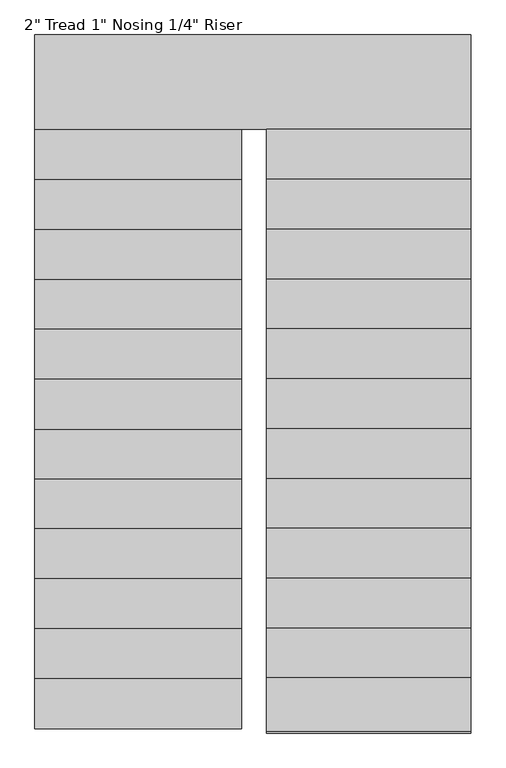
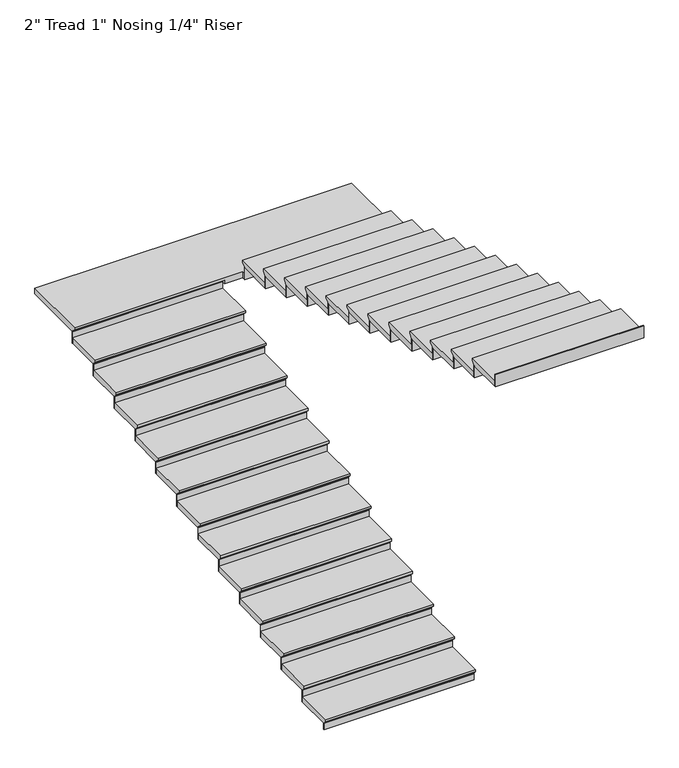
"""IFC4 building model written with IfcOpenShell, lengths in millimetres: stair flight geometry."""

from ifc_helpers import new_model, si_unit, origin, place, context, project, spatial, faceted_brep, source, transform, mapped, element, save


def stair_flight_ff411a25(model_context):
    return source(origin(), model_context, "Body", "Brep", [
        faceted_brep([(-2593.7381751, -9955.5916506, 9230.4576923), (-2593.7381751, -9955.5916506, 9249.5076923), (-3857.687215, -9955.5916506, 9249.5076923), (-3857.687215, -9955.5916506, 9230.4576923), (-2593.7381751, -9930.1916506, 9205.0576923), (-3857.687215, -9930.1916506, 9205.0576923), (-2593.7381751, -9619.0416506, 9249.5076923), (-3857.687215, -9619.0416506, 9249.5076923), (-3857.687215, -9930.1916506, 9198.7076923), (-3857.687215, -9619.0416506, 9198.7076923), (-2593.7381751, -9619.0416506, 9198.7076923), (-2593.7381751, -9930.1916506, 9198.7076923)], [[[0, 1, 2, 3]], [[4, 0, 3, 5]], [[2, 1, 6, 7]], [[8, 9, 10, 11]], [[2, 7, 9, 8, 5, 3]], [[8, 11, 4, 5]], [[6, 1, 0, 4, 11, 10]], [[7, 6, 10, 9]]]),
        faceted_brep([(-2593.7381751, -9930.1916506, 9198.7076923), (-2593.7381751, -9930.1916506, 9144.0), (-2593.7381751, -9923.8416506, 9144.0), (-2593.7381751, -9923.8416506, 9198.7076923), (-3857.687215, -9930.1916506, 9198.7076923), (-3857.687215, -9923.8416506, 9198.7076923), (-3857.687215, -9923.8416506, 9144.0), (-3857.687215, -9930.1916506, 9144.0)], [[[0, 1, 2, 3]], [[4, 5, 6, 7]], [[1, 0, 4, 7]], [[2, 1, 7, 6]], [[3, 2, 6, 5]], [[0, 3, 5, 4]]]),
        faceted_brep([(-2593.7381751, -9619.0416506, 9304.2153846), (-2593.7381751, -9619.0416506, 9198.7076923), (-2593.7381751, -9612.6916506, 9198.7076923), (-2593.7381751, -9612.6916506, 9304.2153846), (-3857.687215, -9619.0416506, 9304.2153846), (-3857.687215, -9612.6916506, 9304.2153846), (-3857.687215, -9612.6916506, 9198.7076923), (-3857.687215, -9619.0416506, 9198.7076923)], [[[0, 1, 2, 3]], [[4, 5, 6, 7]], [[1, 0, 4, 7]], [[2, 1, 7, 6]], [[3, 2, 6, 5]], [[0, 3, 5, 4]]]),
        faceted_brep([(-3857.687215, -9644.4416506, 9355.0153846), (-2593.7381751, -9644.4416506, 9355.0153846), (-2593.7381751, -9314.2416506, 9355.0153846), (-3857.687215, -9314.2416506, 9355.0153846), (-3857.687215, -9619.0416506, 9304.2153846), (-3857.687215, -9314.2416506, 9304.2153846), (-2593.7381751, -9314.2416506, 9304.2153846), (-2593.7381751, -9619.0416506, 9304.2153846), (-3857.687215, -9619.0416506, 9310.5653846), (-3857.687215, -9644.4416506, 9335.9653846), (-2593.7381751, -9619.0416506, 9310.5653846), (-2593.7381751, -9644.4416506, 9335.9653846)], [[[0, 1, 2, 3]], [[4, 5, 6, 7]], [[0, 3, 5, 4, 8, 9]], [[4, 7, 10, 8]], [[2, 1, 11, 10, 7, 6]], [[3, 2, 6, 5]], [[11, 1, 0, 9]], [[10, 11, 9, 8]]]),
        faceted_brep([(-2593.7381751, -9314.2416506, 9409.7230769), (-2593.7381751, -9314.2416506, 9304.2153846), (-2593.7381751, -9307.8916506, 9304.2153846), (-2593.7381751, -9307.8916506, 9409.7230769), (-3857.687215, -9314.2416506, 9409.7230769), (-3857.687215, -9307.8916506, 9409.7230769), (-3857.687215, -9307.8916506, 9304.2153846), (-3857.687215, -9314.2416506, 9304.2153846)], [[[0, 1, 2, 3]], [[4, 5, 6, 7]], [[1, 0, 4, 7]], [[2, 1, 7, 6]], [[3, 2, 6, 5]], [[0, 3, 5, 4]]]),
        faceted_brep([(-3857.687215, -9339.6416506, 9460.5230769), (-2593.7381751, -9339.6416506, 9460.5230769), (-2593.7381751, -9009.4416506, 9460.5230769), (-3857.687215, -9009.4416506, 9460.5230769), (-3857.687215, -9314.2416506, 9409.7230769), (-3857.687215, -9009.4416506, 9409.7230769), (-2593.7381751, -9009.4416506, 9409.7230769), (-2593.7381751, -9314.2416506, 9409.7230769), (-3857.687215, -9314.2416506, 9416.0730769), (-3857.687215, -9339.6416506, 9441.4730769), (-2593.7381751, -9314.2416506, 9416.0730769), (-2593.7381751, -9339.6416506, 9441.4730769)], [[[0, 1, 2, 3]], [[4, 5, 6, 7]], [[0, 3, 5, 4, 8, 9]], [[4, 7, 10, 8]], [[2, 1, 11, 10, 7, 6]], [[3, 2, 6, 5]], [[11, 1, 0, 9]], [[10, 11, 9, 8]]]),
        faceted_brep([(-2593.7381751, -9009.4416506, 9515.2307692), (-2593.7381751, -9009.4416506, 9409.7230769), (-2593.7381751, -9003.0916506, 9409.7230769), (-2593.7381751, -9003.0916506, 9515.2307692), (-3857.687215, -9009.4416506, 9515.2307692), (-3857.687215, -9003.0916506, 9515.2307692), (-3857.687215, -9003.0916506, 9409.7230769), (-3857.687215, -9009.4416506, 9409.7230769)], [[[0, 1, 2, 3]], [[4, 5, 6, 7]], [[1, 0, 4, 7]], [[2, 1, 7, 6]], [[3, 2, 6, 5]], [[0, 3, 5, 4]]]),
        faceted_brep([(-3857.687215, -9034.8416506, 9566.0307692), (-2593.7381751, -9034.8416506, 9566.0307692), (-2593.7381751, -8704.6416506, 9566.0307692), (-3857.687215, -8704.6416506, 9566.0307692), (-3857.687215, -9009.4416506, 9515.2307692), (-3857.687215, -8704.6416506, 9515.2307692), (-2593.7381751, -8704.6416506, 9515.2307692), (-2593.7381751, -9009.4416506, 9515.2307692), (-3857.687215, -9009.4416506, 9521.5807692), (-3857.687215, -9034.8416506, 9546.9807692), (-2593.7381751, -9009.4416506, 9521.5807692), (-2593.7381751, -9034.8416506, 9546.9807692)], [[[0, 1, 2, 3]], [[4, 5, 6, 7]], [[0, 3, 5, 4, 8, 9]], [[4, 7, 10, 8]], [[2, 1, 11, 10, 7, 6]], [[3, 2, 6, 5]], [[11, 1, 0, 9]], [[10, 11, 9, 8]]]),
        faceted_brep([(-2593.7381751, -8704.6416506, 9620.7384615), (-2593.7381751, -8704.6416506, 9515.2307692), (-2593.7381751, -8698.2916506, 9515.2307692), (-2593.7381751, -8698.2916506, 9620.7384615), (-3857.687215, -8704.6416506, 9620.7384615), (-3857.687215, -8698.2916506, 9620.7384615), (-3857.687215, -8698.2916506, 9515.2307692), (-3857.687215, -8704.6416506, 9515.2307692)], [[[0, 1, 2, 3]], [[4, 5, 6, 7]], [[1, 0, 4, 7]], [[2, 1, 7, 6]], [[3, 2, 6, 5]], [[0, 3, 5, 4]]]),
        faceted_brep([(-3857.687215, -8730.0416506, 9671.5384615), (-2593.7381751, -8730.0416506, 9671.5384615), (-2593.7381751, -8399.8416506, 9671.5384615), (-3857.687215, -8399.8416506, 9671.5384615), (-3857.687215, -8704.6416506, 9620.7384615), (-3857.687215, -8399.8416506, 9620.7384615), (-2593.7381751, -8399.8416506, 9620.7384615), (-2593.7381751, -8704.6416506, 9620.7384615), (-3857.687215, -8704.6416506, 9627.0884615), (-3857.687215, -8730.0416506, 9652.4884615), (-2593.7381751, -8704.6416506, 9627.0884615), (-2593.7381751, -8730.0416506, 9652.4884615)], [[[0, 1, 2, 3]], [[4, 5, 6, 7]], [[0, 3, 5, 4, 8, 9]], [[4, 7, 10, 8]], [[2, 1, 11, 10, 7, 6]], [[3, 2, 6, 5]], [[11, 1, 0, 9]], [[10, 11, 9, 8]]]),
        faceted_brep([(-2593.7381751, -8399.8416506, 9726.2461538), (-2593.7381751, -8399.8416506, 9620.7384615), (-2593.7381751, -8393.4916506, 9620.7384615), (-2593.7381751, -8393.4916506, 9726.2461538), (-3857.687215, -8399.8416506, 9726.2461538), (-3857.687215, -8393.4916506, 9726.2461538), (-3857.687215, -8393.4916506, 9620.7384615), (-3857.687215, -8399.8416506, 9620.7384615)], [[[0, 1, 2, 3]], [[4, 5, 6, 7]], [[1, 0, 4, 7]], [[2, 1, 7, 6]], [[3, 2, 6, 5]], [[0, 3, 5, 4]]]),
        faceted_brep([(-3857.687215, -8425.2416506, 9777.0461538), (-2593.7381751, -8425.2416506, 9777.0461538), (-2593.7381751, -8098.2166506, 9777.0461538), (-3857.687215, -8098.2166506, 9777.0461538), (-3857.687215, -8399.8416506, 9726.2461538), (-3857.687215, -8098.2166506, 9726.2461538), (-2593.7381751, -8098.2166506, 9726.2461538), (-2593.7381751, -8399.8416506, 9726.2461538), (-3857.687215, -8399.8416506, 9732.5961538), (-3857.687215, -8425.2416506, 9757.9961538), (-2593.7381751, -8399.8416506, 9732.5961538), (-2593.7381751, -8425.2416506, 9757.9961538)], [[[0, 1, 2, 3]], [[4, 5, 6, 7]], [[0, 3, 5, 4, 8, 9]], [[4, 7, 10, 8]], [[2, 1, 11, 10, 7, 6]], [[3, 2, 6, 5]], [[11, 1, 0, 9]], [[10, 11, 9, 8]]]),
        faceted_brep([(-2593.7381751, -8098.2166506, 9831.7538462), (-2593.7381751, -8098.2166506, 9726.2461538), (-2593.7381751, -8091.8666506, 9726.2461538), (-2593.7381751, -8091.8666506, 9831.7538462), (-3857.687215, -8098.2166506, 9831.7538462), (-3857.687215, -8091.8666506, 9831.7538462), (-3857.687215, -8091.8666506, 9726.2461538), (-3857.687215, -8098.2166506, 9726.2461538)], [[[0, 1, 2, 3]], [[4, 5, 6, 7]], [[1, 0, 4, 7]], [[2, 1, 7, 6]], [[3, 2, 6, 5]], [[0, 3, 5, 4]]]),
        faceted_brep([(-3857.687215, -8123.6166506, 9882.5538462), (-2593.7381751, -8123.6166506, 9882.5538462), (-2593.7381751, -7790.2416506, 9882.5538462), (-3857.687215, -7790.2416506, 9882.5538462), (-3857.687215, -8098.2166506, 9831.7538462), (-3857.687215, -7790.2416506, 9831.7538462), (-2593.7381751, -7790.2416506, 9831.7538462), (-2593.7381751, -8098.2166506, 9831.7538462), (-3857.687215, -8098.2166506, 9838.1038462), (-3857.687215, -8123.6166506, 9863.5038462), (-2593.7381751, -8098.2166506, 9838.1038462), (-2593.7381751, -8123.6166506, 9863.5038462)], [[[0, 1, 2, 3]], [[4, 5, 6, 7]], [[0, 3, 5, 4, 8, 9]], [[4, 7, 10, 8]], [[2, 1, 11, 10, 7, 6]], [[3, 2, 6, 5]], [[11, 1, 0, 9]], [[10, 11, 9, 8]]]),
        faceted_brep([(-2593.7381751, -7790.2416506, 9937.2615385), (-2593.7381751, -7790.2416506, 9831.7538462), (-2593.7381751, -7783.8916506, 9831.7538462), (-2593.7381751, -7783.8916506, 9937.2615385), (-3857.687215, -7790.2416506, 9937.2615385), (-3857.687215, -7783.8916506, 9937.2615385), (-3857.687215, -7783.8916506, 9831.7538462), (-3857.687215, -7790.2416506, 9831.7538462)], [[[0, 1, 2, 3]], [[4, 5, 6, 7]], [[1, 0, 4, 7]], [[2, 1, 7, 6]], [[3, 2, 6, 5]], [[0, 3, 5, 4]]]),
        faceted_brep([(-3857.687215, -7815.6416506, 9988.0615385), (-2593.7381751, -7815.6416506, 9988.0615385), (-2593.7381751, -7485.4416506, 9988.0615385), (-3857.687215, -7485.4416506, 9988.0615385), (-3857.687215, -7790.2416506, 9937.2615385), (-3857.687215, -7485.4416506, 9937.2615385), (-2593.7381751, -7485.4416506, 9937.2615385), (-2593.7381751, -7790.2416506, 9937.2615385), (-3857.687215, -7790.2416506, 9943.6115385), (-3857.687215, -7815.6416506, 9969.0115385), (-2593.7381751, -7790.2416506, 9943.6115385), (-2593.7381751, -7815.6416506, 9969.0115385)], [[[0, 1, 2, 3]], [[4, 5, 6, 7]], [[0, 3, 5, 4, 8, 9]], [[4, 7, 10, 8]], [[2, 1, 11, 10, 7, 6]], [[3, 2, 6, 5]], [[11, 1, 0, 9]], [[10, 11, 9, 8]]]),
        faceted_brep([(-2593.7381751, -7485.4416506, 10042.7692308), (-2593.7381751, -7485.4416506, 9937.2615385), (-2593.7381751, -7479.0916506, 9937.2615385), (-2593.7381751, -7479.0916506, 10042.7692308), (-3857.687215, -7485.4416506, 10042.7692308), (-3857.687215, -7479.0916506, 10042.7692308), (-3857.687215, -7479.0916506, 9937.2615385), (-3857.687215, -7485.4416506, 9937.2615385)], [[[0, 1, 2, 3]], [[4, 5, 6, 7]], [[1, 0, 4, 7]], [[2, 1, 7, 6]], [[3, 2, 6, 5]], [[0, 3, 5, 4]]]),
        faceted_brep([(-3857.687215, -7510.8416506, 10093.5692308), (-2593.7381751, -7510.8416506, 10093.5692308), (-2593.7381751, -7180.6416506, 10093.5692308), (-3857.687215, -7180.6416506, 10093.5692308), (-3857.687215, -7485.4416506, 10042.7692308), (-3857.687215, -7180.6416506, 10042.7692308), (-2593.7381751, -7180.6416506, 10042.7692308), (-2593.7381751, -7485.4416506, 10042.7692308), (-3857.687215, -7485.4416506, 10049.1192308), (-3857.687215, -7510.8416506, 10074.5192308), (-2593.7381751, -7485.4416506, 10049.1192308), (-2593.7381751, -7510.8416506, 10074.5192308)], [[[0, 1, 2, 3]], [[4, 5, 6, 7]], [[0, 3, 5, 4, 8, 9]], [[4, 7, 10, 8]], [[2, 1, 11, 10, 7, 6]], [[3, 2, 6, 5]], [[11, 1, 0, 9]], [[10, 11, 9, 8]]]),
        faceted_brep([(-2593.7381751, -7180.6416506, 10148.2769231), (-2593.7381751, -7180.6416506, 10042.7692308), (-2593.7381751, -7174.2916506, 10042.7692308), (-2593.7381751, -7174.2916506, 10148.2769231), (-3857.687215, -7180.6416506, 10148.2769231), (-3857.687215, -7174.2916506, 10148.2769231), (-3857.687215, -7174.2916506, 10042.7692308), (-3857.687215, -7180.6416506, 10042.7692308)], [[[0, 1, 2, 3]], [[4, 5, 6, 7]], [[1, 0, 4, 7]], [[2, 1, 7, 6]], [[3, 2, 6, 5]], [[0, 3, 5, 4]]]),
        faceted_brep([(-3857.687215, -7206.0416506, 10199.0769231), (-2593.7381751, -7206.0416506, 10199.0769231), (-2593.7381751, -6875.8416506, 10199.0769231), (-3857.687215, -6875.8416506, 10199.0769231), (-3857.687215, -7180.6416506, 10148.2769231), (-3857.687215, -6875.8416506, 10148.2769231), (-2593.7381751, -6875.8416506, 10148.2769231), (-2593.7381751, -7180.6416506, 10148.2769231), (-3857.687215, -7180.6416506, 10154.6269231), (-3857.687215, -7206.0416506, 10180.0269231), (-2593.7381751, -7180.6416506, 10154.6269231), (-2593.7381751, -7206.0416506, 10180.0269231)], [[[0, 1, 2, 3]], [[4, 5, 6, 7]], [[0, 3, 5, 4, 8, 9]], [[4, 7, 10, 8]], [[2, 1, 11, 10, 7, 6]], [[3, 2, 6, 5]], [[11, 1, 0, 9]], [[10, 11, 9, 8]]]),
        faceted_brep([(-2593.7381751, -6875.8416506, 10253.7846154), (-2593.7381751, -6875.8416506, 10148.2769231), (-2593.7381751, -6869.4916506, 10148.2769231), (-2593.7381751, -6869.4916506, 10253.7846154), (-3857.687215, -6875.8416506, 10253.7846154), (-3857.687215, -6869.4916506, 10253.7846154), (-3857.687215, -6869.4916506, 10148.2769231), (-3857.687215, -6875.8416506, 10148.2769231)], [[[0, 1, 2, 3]], [[4, 5, 6, 7]], [[1, 0, 4, 7]], [[2, 1, 7, 6]], [[3, 2, 6, 5]], [[0, 3, 5, 4]]]),
        faceted_brep([(-3857.687215, -6901.2416506, 10304.5846154), (-2593.7381751, -6901.2416506, 10304.5846154), (-2593.7381751, -6571.0416506, 10304.5846154), (-3857.687215, -6571.0416506, 10304.5846154), (-3857.687215, -6875.8416506, 10253.7846154), (-3857.687215, -6571.0416506, 10253.7846154), (-2593.7381751, -6571.0416506, 10253.7846154), (-2593.7381751, -6875.8416506, 10253.7846154), (-3857.687215, -6875.8416506, 10260.1346154), (-3857.687215, -6901.2416506, 10285.5346154), (-2593.7381751, -6875.8416506, 10260.1346154), (-2593.7381751, -6901.2416506, 10285.5346154)], [[[0, 1, 2, 3]], [[4, 5, 6, 7]], [[0, 3, 5, 4, 8, 9]], [[4, 7, 10, 8]], [[2, 1, 11, 10, 7, 6]], [[3, 2, 6, 5]], [[11, 1, 0, 9]], [[10, 11, 9, 8]]]),
        faceted_brep([(-2593.7381751, -6571.0416506, 10359.2923077), (-2593.7381751, -6571.0416506, 10253.7846154), (-2593.7381751, -6564.6916506, 10253.7846154), (-2593.7381751, -6564.6916506, 10359.2923077), (-3857.687215, -6571.0416506, 10359.2923077), (-3857.687215, -6564.6916506, 10359.2923077), (-3857.687215, -6564.6916506, 10253.7846154), (-3857.687215, -6571.0416506, 10253.7846154)], [[[0, 1, 2, 3]], [[4, 5, 6, 7]], [[1, 0, 4, 7]], [[2, 1, 7, 6]], [[3, 2, 6, 5]], [[0, 3, 5, 4]]]),
        faceted_brep([(-3857.687215, -6596.4416506, 10410.0923077), (-2593.7381751, -6596.4416506, 10410.0923077), (-2593.7381751, -6266.2416506, 10410.0923077), (-3857.687215, -6266.2416506, 10410.0923077), (-3857.687215, -6571.0416506, 10359.2923077), (-3857.687215, -6266.2416506, 10359.2923077), (-2593.7381751, -6266.2416506, 10359.2923077), (-2593.7381751, -6571.0416506, 10359.2923077), (-3857.687215, -6571.0416506, 10365.6423077), (-3857.687215, -6596.4416506, 10391.0423077), (-2593.7381751, -6571.0416506, 10365.6423077), (-2593.7381751, -6596.4416506, 10391.0423077)], [[[0, 1, 2, 3]], [[4, 5, 6, 7]], [[0, 3, 5, 4, 8, 9]], [[4, 7, 10, 8]], [[2, 1, 11, 10, 7, 6]], [[3, 2, 6, 5]], [[11, 1, 0, 9]], [[10, 11, 9, 8]]]),
        faceted_brep([(-2593.7381751, -6266.2416506, 10464.8), (-2593.7381751, -6266.2416506, 10359.2923077), (-2593.7381751, -6259.8916506, 10359.2923077), (-2593.7381751, -6259.8916506, 10464.8), (-3857.687215, -6266.2416506, 10464.8), (-3857.687215, -6259.8916506, 10464.8), (-3857.687215, -6259.8916506, 10359.2923077), (-3857.687215, -6266.2416506, 10359.2923077)], [[[0, 1, 2, 3]], [[4, 5, 6, 7]], [[1, 0, 4, 7]], [[2, 1, 7, 6]], [[3, 2, 6, 5]], [[0, 3, 5, 4]]]),
        faceted_brep([(-1190.687215, -6317.0416506, 10515.6), (-1190.687215, -5713.7916506, 10515.6), (-3857.687215, -5713.7916506, 10515.6), (-3857.687215, -6291.6416506, 10515.6), (-2441.3381751, -6291.6416506, 10515.6), (-2441.3381751, -6317.0416506, 10515.6), (-1190.687215, -5713.7916506, 10464.8), (-1190.687215, -6317.0416506, 10464.8), (-2441.3381751, -6317.0416506, 10464.8), (-2441.3381751, -6291.6416506, 10464.8), (-2593.7381751, -6291.6416506, 10464.8), (-2593.7381751, -6266.2416506, 10464.8), (-3857.687215, -6266.2416506, 10464.8), (-3857.687215, -5713.7916506, 10464.8), (-3857.687215, -6266.2416506, 10471.15), (-3857.687215, -6291.6416506, 10496.55), (-2593.7381751, -6266.2416506, 10471.15), (-2593.7381751, -6291.6416506, 10496.55)], [[[0, 1, 2, 3, 4, 5]], [[6, 7, 8, 9, 10, 11, 12, 13]], [[1, 0, 7, 6]], [[2, 1, 6, 13]], [[3, 2, 13, 12, 14, 15]], [[12, 11, 16, 14]], [[11, 10, 17, 16]], [[4, 3, 15, 17, 10, 9]], [[5, 4, 9, 8]], [[0, 5, 8, 7]], [[15, 14, 16, 17]]]),
        faceted_brep([(-2441.3381751, -6317.0416506, 10570.3076923), (-2441.3381751, -6317.0416506, 10464.8), (-2441.3381751, -6323.3916506, 10464.8), (-2441.3381751, -6323.3916506, 10570.3076923), (-1190.687215, -6317.0416506, 10570.3076923), (-1190.687215, -6323.3916506, 10570.3076923), (-1190.687215, -6323.3916506, 10464.8), (-1190.687215, -6317.0416506, 10464.8)], [[[0, 1, 2, 3]], [[4, 5, 6, 7]], [[1, 0, 4, 7]], [[2, 1, 7, 6]], [[3, 2, 6, 5]], [[0, 3, 5, 4]]]),
        faceted_brep([(-1190.687215, -6291.6416506, 10621.1076923), (-2441.3381751, -6291.6416506, 10621.1076923), (-2441.3381751, -6621.8416506, 10621.1076923), (-1190.687215, -6621.8416506, 10621.1076923), (-1190.687215, -6317.0416506, 10570.3076923), (-1190.687215, -6621.8416506, 10570.3076923), (-2441.3381751, -6621.8416506, 10570.3076923), (-2441.3381751, -6317.0416506, 10570.3076923), (-1190.687215, -6317.0416506, 10576.6576923), (-1190.687215, -6291.6416506, 10602.0576923), (-2441.3381751, -6317.0416506, 10576.6576923), (-2441.3381751, -6291.6416506, 10602.0576923)], [[[0, 1, 2, 3]], [[4, 5, 6, 7]], [[0, 3, 5, 4, 8, 9]], [[4, 7, 10, 8]], [[2, 1, 11, 10, 7, 6]], [[3, 2, 6, 5]], [[11, 1, 0, 9]], [[10, 11, 9, 8]]]),
        faceted_brep([(-2441.3381751, -6621.8416506, 10675.8153846), (-2441.3381751, -6621.8416506, 10570.3076923), (-2441.3381751, -6628.1916506, 10570.3076923), (-2441.3381751, -6628.1916506, 10675.8153846), (-1190.687215, -6621.8416506, 10675.8153846), (-1190.687215, -6628.1916506, 10675.8153846), (-1190.687215, -6628.1916506, 10570.3076923), (-1190.687215, -6621.8416506, 10570.3076923)], [[[0, 1, 2, 3]], [[4, 5, 6, 7]], [[1, 0, 4, 7]], [[2, 1, 7, 6]], [[3, 2, 6, 5]], [[0, 3, 5, 4]]]),
        faceted_brep([(-1190.687215, -6596.4416506, 10726.6153846), (-2441.3381751, -6596.4416506, 10726.6153846), (-2441.3381751, -6926.6416506, 10726.6153846), (-1190.687215, -6926.6416506, 10726.6153846), (-1190.687215, -6621.8416506, 10675.8153846), (-1190.687215, -6926.6416506, 10675.8153846), (-2441.3381751, -6926.6416506, 10675.8153846), (-2441.3381751, -6621.8416506, 10675.8153846), (-1190.687215, -6621.8416506, 10682.1653846), (-1190.687215, -6596.4416506, 10707.5653846), (-2441.3381751, -6621.8416506, 10682.1653846), (-2441.3381751, -6596.4416506, 10707.5653846)], [[[0, 1, 2, 3]], [[4, 5, 6, 7]], [[0, 3, 5, 4, 8, 9]], [[4, 7, 10, 8]], [[2, 1, 11, 10, 7, 6]], [[3, 2, 6, 5]], [[11, 1, 0, 9]], [[10, 11, 9, 8]]]),
        faceted_brep([(-2441.3381751, -6926.6416506, 10781.3230769), (-2441.3381751, -6926.6416506, 10675.8153846), (-2441.3381751, -6932.9916506, 10675.8153846), (-2441.3381751, -6932.9916506, 10781.3230769), (-1190.687215, -6926.6416506, 10781.3230769), (-1190.687215, -6932.9916506, 10781.3230769), (-1190.687215, -6932.9916506, 10675.8153846), (-1190.687215, -6926.6416506, 10675.8153846)], [[[0, 1, 2, 3]], [[4, 5, 6, 7]], [[1, 0, 4, 7]], [[2, 1, 7, 6]], [[3, 2, 6, 5]], [[0, 3, 5, 4]]]),
        faceted_brep([(-1190.687215, -6901.2416506, 10832.1230769), (-2441.3381751, -6901.2416506, 10832.1230769), (-2441.3381751, -7231.4416506, 10832.1230769), (-1190.687215, -7231.4416506, 10832.1230769), (-1190.687215, -6926.6416506, 10781.3230769), (-1190.687215, -7231.4416506, 10781.3230769), (-2441.3381751, -7231.4416506, 10781.3230769), (-2441.3381751, -6926.6416506, 10781.3230769), (-1190.687215, -6926.6416506, 10787.6730769), (-1190.687215, -6901.2416506, 10813.0730769), (-2441.3381751, -6926.6416506, 10787.6730769), (-2441.3381751, -6901.2416506, 10813.0730769)], [[[0, 1, 2, 3]], [[4, 5, 6, 7]], [[0, 3, 5, 4, 8, 9]], [[4, 7, 10, 8]], [[2, 1, 11, 10, 7, 6]], [[3, 2, 6, 5]], [[11, 1, 0, 9]], [[10, 11, 9, 8]]]),
        faceted_brep([(-2441.3381751, -7231.4416506, 10886.8307692), (-2441.3381751, -7231.4416506, 10781.3230769), (-2441.3381751, -7237.7916506, 10781.3230769), (-2441.3381751, -7237.7916506, 10886.8307692), (-1190.687215, -7231.4416506, 10886.8307692), (-1190.687215, -7237.7916506, 10886.8307692), (-1190.687215, -7237.7916506, 10781.3230769), (-1190.687215, -7231.4416506, 10781.3230769)], [[[0, 1, 2, 3]], [[4, 5, 6, 7]], [[1, 0, 4, 7]], [[2, 1, 7, 6]], [[3, 2, 6, 5]], [[0, 3, 5, 4]]]),
        faceted_brep([(-1190.687215, -7206.0416506, 10937.6307692), (-2441.3381751, -7206.0416506, 10937.6307692), (-2441.3381751, -7536.2416506, 10937.6307692), (-1190.687215, -7536.2416506, 10937.6307692), (-1190.687215, -7231.4416506, 10886.8307692), (-1190.687215, -7536.2416506, 10886.8307692), (-2441.3381751, -7536.2416506, 10886.8307692), (-2441.3381751, -7231.4416506, 10886.8307692), (-1190.687215, -7231.4416506, 10893.1807692), (-1190.687215, -7206.0416506, 10918.5807692), (-2441.3381751, -7231.4416506, 10893.1807692), (-2441.3381751, -7206.0416506, 10918.5807692)], [[[0, 1, 2, 3]], [[4, 5, 6, 7]], [[0, 3, 5, 4, 8, 9]], [[4, 7, 10, 8]], [[2, 1, 11, 10, 7, 6]], [[3, 2, 6, 5]], [[11, 1, 0, 9]], [[10, 11, 9, 8]]]),
        faceted_brep([(-2441.3381751, -7536.2416506, 10992.3384615), (-2441.3381751, -7536.2416506, 10886.8307692), (-2441.3381751, -7542.5916506, 10886.8307692), (-2441.3381751, -7542.5916506, 10992.3384615), (-1190.687215, -7536.2416506, 10992.3384615), (-1190.687215, -7542.5916506, 10992.3384615), (-1190.687215, -7542.5916506, 10886.8307692), (-1190.687215, -7536.2416506, 10886.8307692)], [[[0, 1, 2, 3]], [[4, 5, 6, 7]], [[1, 0, 4, 7]], [[2, 1, 7, 6]], [[3, 2, 6, 5]], [[0, 3, 5, 4]]]),
        faceted_brep([(-1190.687215, -7510.8416506, 11043.1384615), (-2441.3381751, -7510.8416506, 11043.1384615), (-2441.3381751, -7841.0416506, 11043.1384615), (-1190.687215, -7841.0416506, 11043.1384615), (-1190.687215, -7536.2416506, 10992.3384615), (-1190.687215, -7841.0416506, 10992.3384615), (-2441.3381751, -7841.0416506, 10992.3384615), (-2441.3381751, -7536.2416506, 10992.3384615), (-1190.687215, -7536.2416506, 10998.6884615), (-1190.687215, -7510.8416506, 11024.0884615), (-2441.3381751, -7536.2416506, 10998.6884615), (-2441.3381751, -7510.8416506, 11024.0884615)], [[[0, 1, 2, 3]], [[4, 5, 6, 7]], [[0, 3, 5, 4, 8, 9]], [[4, 7, 10, 8]], [[2, 1, 11, 10, 7, 6]], [[3, 2, 6, 5]], [[11, 1, 0, 9]], [[10, 11, 9, 8]]]),
        faceted_brep([(-2441.3381751, -7841.0416506, 11097.8461538), (-2441.3381751, -7841.0416506, 10992.3384615), (-2441.3381751, -7847.3916506, 10992.3384615), (-2441.3381751, -7847.3916506, 11097.8461538), (-1190.687215, -7841.0416506, 11097.8461538), (-1190.687215, -7847.3916506, 11097.8461538), (-1190.687215, -7847.3916506, 10992.3384615), (-1190.687215, -7841.0416506, 10992.3384615)], [[[0, 1, 2, 3]], [[4, 5, 6, 7]], [[1, 0, 4, 7]], [[2, 1, 7, 6]], [[3, 2, 6, 5]], [[0, 3, 5, 4]]]),
        faceted_brep([(-1190.687215, -7815.6416506, 11148.6461538), (-2441.3381751, -7815.6416506, 11148.6461538), (-2441.3381751, -8145.8416506, 11148.6461538), (-1190.687215, -8145.8416506, 11148.6461538), (-1190.687215, -7841.0416506, 11097.8461538), (-1190.687215, -8145.8416506, 11097.8461538), (-2441.3381751, -8145.8416506, 11097.8461538), (-2441.3381751, -7841.0416506, 11097.8461538), (-1190.687215, -7841.0416506, 11104.1961538), (-1190.687215, -7815.6416506, 11129.5961538), (-2441.3381751, -7841.0416506, 11104.1961538), (-2441.3381751, -7815.6416506, 11129.5961538)], [[[0, 1, 2, 3]], [[4, 5, 6, 7]], [[0, 3, 5, 4, 8, 9]], [[4, 7, 10, 8]], [[2, 1, 11, 10, 7, 6]], [[3, 2, 6, 5]], [[11, 1, 0, 9]], [[10, 11, 9, 8]]]),
        faceted_brep([(-2441.3381751, -8145.8416506, 11203.3538462), (-2441.3381751, -8145.8416506, 11097.8461538), (-2441.3381751, -8152.1916506, 11097.8461538), (-2441.3381751, -8152.1916506, 11203.3538462), (-1190.687215, -8145.8416506, 11203.3538462), (-1190.687215, -8152.1916506, 11203.3538462), (-1190.687215, -8152.1916506, 11097.8461538), (-1190.687215, -8145.8416506, 11097.8461538)], [[[0, 1, 2, 3]], [[4, 5, 6, 7]], [[1, 0, 4, 7]], [[2, 1, 7, 6]], [[3, 2, 6, 5]], [[0, 3, 5, 4]]]),
        faceted_brep([(-1190.687215, -8120.4416506, 11254.1538462), (-2441.3381751, -8120.4416506, 11254.1538462), (-2441.3381751, -8450.6416506, 11254.1538462), (-1190.687215, -8450.6416506, 11254.1538462), (-1190.687215, -8145.8416506, 11203.3538462), (-1190.687215, -8450.6416506, 11203.3538462), (-2441.3381751, -8450.6416506, 11203.3538462), (-2441.3381751, -8145.8416506, 11203.3538462), (-1190.687215, -8145.8416506, 11209.7038462), (-1190.687215, -8120.4416506, 11235.1038462), (-2441.3381751, -8145.8416506, 11209.7038462), (-2441.3381751, -8120.4416506, 11235.1038462)], [[[0, 1, 2, 3]], [[4, 5, 6, 7]], [[0, 3, 5, 4, 8, 9]], [[4, 7, 10, 8]], [[2, 1, 11, 10, 7, 6]], [[3, 2, 6, 5]], [[11, 1, 0, 9]], [[10, 11, 9, 8]]]),
        faceted_brep([(-2441.3381751, -8450.6416506, 11308.8615385), (-2441.3381751, -8450.6416506, 11203.3538462), (-2441.3381751, -8456.9916506, 11203.3538462), (-2441.3381751, -8456.9916506, 11308.8615385), (-1190.687215, -8450.6416506, 11308.8615385), (-1190.687215, -8456.9916506, 11308.8615385), (-1190.687215, -8456.9916506, 11203.3538462), (-1190.687215, -8450.6416506, 11203.3538462)], [[[0, 1, 2, 3]], [[4, 5, 6, 7]], [[1, 0, 4, 7]], [[2, 1, 7, 6]], [[3, 2, 6, 5]], [[0, 3, 5, 4]]]),
        faceted_brep([(-1190.687215, -8425.2416506, 11359.6615385), (-2441.3381751, -8425.2416506, 11359.6615385), (-2441.3381751, -8755.4416506, 11359.6615385), (-1190.687215, -8755.4416506, 11359.6615385), (-1190.687215, -8450.6416506, 11308.8615385), (-1190.687215, -8755.4416506, 11308.8615385), (-2441.3381751, -8755.4416506, 11308.8615385), (-2441.3381751, -8450.6416506, 11308.8615385), (-1190.687215, -8450.6416506, 11315.2115385), (-1190.687215, -8425.2416506, 11340.6115385), (-2441.3381751, -8450.6416506, 11315.2115385), (-2441.3381751, -8425.2416506, 11340.6115385)], [[[0, 1, 2, 3]], [[4, 5, 6, 7]], [[0, 3, 5, 4, 8, 9]], [[4, 7, 10, 8]], [[2, 1, 11, 10, 7, 6]], [[3, 2, 6, 5]], [[11, 1, 0, 9]], [[10, 11, 9, 8]]]),
        faceted_brep([(-2441.3381751, -8755.4416506, 11414.3692308), (-2441.3381751, -8755.4416506, 11308.8615385), (-2441.3381751, -8761.7916506, 11308.8615385), (-2441.3381751, -8761.7916506, 11414.3692308), (-1190.687215, -8755.4416506, 11414.3692308), (-1190.687215, -8761.7916506, 11414.3692308), (-1190.687215, -8761.7916506, 11308.8615385), (-1190.687215, -8755.4416506, 11308.8615385)], [[[0, 1, 2, 3]], [[4, 5, 6, 7]], [[1, 0, 4, 7]], [[2, 1, 7, 6]], [[3, 2, 6, 5]], [[0, 3, 5, 4]]]),
        faceted_brep([(-1190.687215, -8730.0416506, 11465.1692308), (-2441.3381751, -8730.0416506, 11465.1692308), (-2441.3381751, -9060.2416506, 11465.1692308), (-1190.687215, -9060.2416506, 11465.1692308), (-1190.687215, -8755.4416506, 11414.3692308), (-1190.687215, -9060.2416506, 11414.3692308), (-2441.3381751, -9060.2416506, 11414.3692308), (-2441.3381751, -8755.4416506, 11414.3692308), (-1190.687215, -8755.4416506, 11420.7192308), (-1190.687215, -8730.0416506, 11446.1192308), (-2441.3381751, -8755.4416506, 11420.7192308), (-2441.3381751, -8730.0416506, 11446.1192308)], [[[0, 1, 2, 3]], [[4, 5, 6, 7]], [[0, 3, 5, 4, 8, 9]], [[4, 7, 10, 8]], [[2, 1, 11, 10, 7, 6]], [[3, 2, 6, 5]], [[11, 1, 0, 9]], [[10, 11, 9, 8]]]),
        faceted_brep([(-2441.3381751, -9060.2416506, 11519.8769231), (-2441.3381751, -9060.2416506, 11414.3692308), (-2441.3381751, -9066.5916506, 11414.3692308), (-2441.3381751, -9066.5916506, 11519.8769231), (-1190.687215, -9060.2416506, 11519.8769231), (-1190.687215, -9066.5916506, 11519.8769231), (-1190.687215, -9066.5916506, 11414.3692308), (-1190.687215, -9060.2416506, 11414.3692308)], [[[0, 1, 2, 3]], [[4, 5, 6, 7]], [[1, 0, 4, 7]], [[2, 1, 7, 6]], [[3, 2, 6, 5]], [[0, 3, 5, 4]]]),
        faceted_brep([(-1190.687215, -9034.8416506, 11570.6769231), (-2441.3381751, -9034.8416506, 11570.6769231), (-2441.3381751, -9365.0416506, 11570.6769231), (-1190.687215, -9365.0416506, 11570.6769231), (-1190.687215, -9060.2416506, 11519.8769231), (-1190.687215, -9365.0416506, 11519.8769231), (-2441.3381751, -9365.0416506, 11519.8769231), (-2441.3381751, -9060.2416506, 11519.8769231), (-1190.687215, -9060.2416506, 11526.2269231), (-1190.687215, -9034.8416506, 11551.6269231), (-2441.3381751, -9060.2416506, 11526.2269231), (-2441.3381751, -9034.8416506, 11551.6269231)], [[[0, 1, 2, 3]], [[4, 5, 6, 7]], [[0, 3, 5, 4, 8, 9]], [[4, 7, 10, 8]], [[2, 1, 11, 10, 7, 6]], [[3, 2, 6, 5]], [[11, 1, 0, 9]], [[10, 11, 9, 8]]]),
        faceted_brep([(-2441.3381751, -9365.0416506, 11625.3846154), (-2441.3381751, -9365.0416506, 11519.8769231), (-2441.3381751, -9371.3916506, 11519.8769231), (-2441.3381751, -9371.3916506, 11625.3846154), (-1190.687215, -9365.0416506, 11625.3846154), (-1190.687215, -9371.3916506, 11625.3846154), (-1190.687215, -9371.3916506, 11519.8769231), (-1190.687215, -9365.0416506, 11519.8769231)], [[[0, 1, 2, 3]], [[4, 5, 6, 7]], [[1, 0, 4, 7]], [[2, 1, 7, 6]], [[3, 2, 6, 5]], [[0, 3, 5, 4]]]),
        faceted_brep([(-1190.687215, -9339.6416506, 11676.1846154), (-2441.3381751, -9339.6416506, 11676.1846154), (-2441.3381751, -9669.8416506, 11676.1846154), (-1190.687215, -9669.8416506, 11676.1846154), (-1190.687215, -9365.0416506, 11625.3846154), (-1190.687215, -9669.8416506, 11625.3846154), (-2441.3381751, -9669.8416506, 11625.3846154), (-2441.3381751, -9365.0416506, 11625.3846154), (-1190.687215, -9365.0416506, 11631.7346154), (-1190.687215, -9339.6416506, 11657.1346154), (-2441.3381751, -9365.0416506, 11631.7346154), (-2441.3381751, -9339.6416506, 11657.1346154)], [[[0, 1, 2, 3]], [[4, 5, 6, 7]], [[0, 3, 5, 4, 8, 9]], [[4, 7, 10, 8]], [[2, 1, 11, 10, 7, 6]], [[3, 2, 6, 5]], [[11, 1, 0, 9]], [[10, 11, 9, 8]]]),
        faceted_brep([(-2441.3381751, -9669.8416506, 11730.8923077), (-2441.3381751, -9669.8416506, 11625.3846154), (-2441.3381751, -9676.1916506, 11625.3846154), (-2441.3381751, -9676.1916506, 11730.8923077), (-1190.687215, -9669.8416506, 11730.8923077), (-1190.687215, -9676.1916506, 11730.8923077), (-1190.687215, -9676.1916506, 11625.3846154), (-1190.687215, -9669.8416506, 11625.3846154)], [[[0, 1, 2, 3]], [[4, 5, 6, 7]], [[1, 0, 4, 7]], [[2, 1, 7, 6]], [[3, 2, 6, 5]], [[0, 3, 5, 4]]]),
        faceted_brep([(-2441.3381751, -9974.6416506, 11836.4), (-2441.3381751, -9974.6416506, 11730.8923077), (-2441.3381751, -9980.9916506, 11730.8923077), (-2441.3381751, -9980.9916506, 11836.4), (-1190.687215, -9974.6416506, 11836.4), (-1190.687215, -9980.9916506, 11836.4), (-1190.687215, -9980.9916506, 11730.8923077), (-1190.687215, -9974.6416506, 11730.8923077)], [[[0, 1, 2, 3]], [[4, 5, 6, 7]], [[1, 0, 4, 7]], [[2, 1, 7, 6]], [[3, 2, 6, 5]], [[0, 3, 5, 4]]]),
        faceted_brep([(-1190.687215, -9644.4416506, 11781.6923077), (-2441.3381751, -9644.4416506, 11781.6923077), (-2441.3381751, -9974.6416506, 11781.6923077), (-1190.687215, -9974.6416506, 11781.6923077), (-1190.687215, -9669.8416506, 11730.8923077), (-1190.687215, -9974.6416506, 11730.8923077), (-2441.3381751, -9974.6416506, 11730.8923077), (-2441.3381751, -9669.8416506, 11730.8923077), (-1190.687215, -9669.8416506, 11737.2423077), (-1190.687215, -9644.4416506, 11762.6423077), (-2441.3381751, -9669.8416506, 11737.2423077), (-2441.3381751, -9644.4416506, 11762.6423077)], [[[0, 1, 2, 3]], [[4, 5, 6, 7]], [[0, 3, 5, 4, 8, 9]], [[4, 7, 10, 8]], [[2, 1, 11, 10, 7, 6]], [[3, 2, 6, 5]], [[11, 1, 0, 9]], [[10, 11, 9, 8]]]),
    ])


if __name__ == "__main__":
    model = new_model("IFC4")
    model_context = context("Model", 3, world=origin())
    ifc_project = project(units=[si_unit("LENGTHUNIT", "METRE", prefix="MILLI")], contexts=[model_context])
    site = spatial("IfcSite", under=ifc_project)
    building = spatial("IfcBuilding", under=site)
    placement = place(None, origin())
    stair_flight_shape = stair_flight_ff411a25(model_context)
    element("IfcStairFlight", 1, ObjectType="2\" Tread 1\" Nosing 1/4\" Riser", at=placement, inside=building, context=model_context, shape_type="MappedRepresentation", body=[
        mapped(stair_flight_shape, transform((0.0, 0.0, 0.0), x_axis=(1.0, 0.0, 0.0), y_axis=(0.0, 1.0, 0.0), z_axis=(0.0, 0.0, 1.0))),
    ])
    save(model, "model.ifc")
